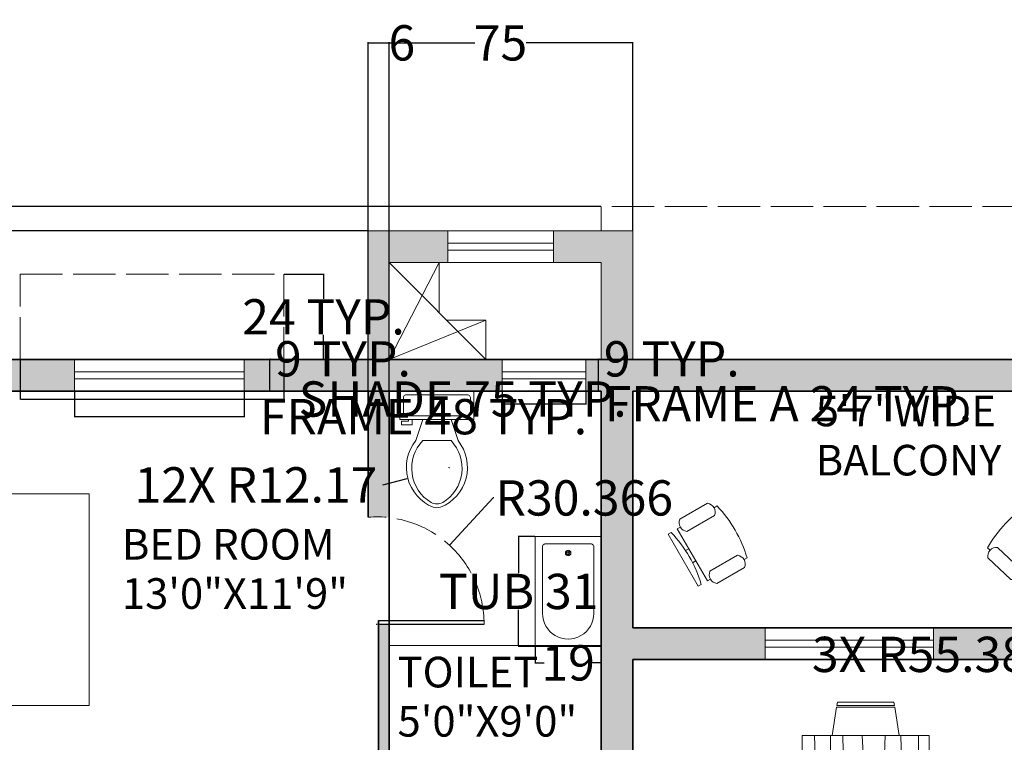
# Model space of a CAD drawing. Units: inches. Extents: x 215 to 969, y -612 to 418.
# Tile 7 of 8: x 405 to 684, y 214 to 418. Entities that reach past the tile are written whole.
import ezdxf

# ---------------------------------------------------------------- set-up
doc = ezdxf.new("R2010")
doc.units = ezdxf.units.IN
doc.header["$MEASUREMENT"] = 0
doc.linetypes.add('ACAD_ISO02W100', pattern=[15, 12, -3])
for name, color, linetype, lineweight in [('A-ANNO-DIMS', 2, 'Continuous', 18), ('A-AREA-IDEN', 7, 'Continuous', 18), ('A-DOOR', 3, 'Continuous', 25), ('A-DOOR-SWNG', 3, 'ACAD_ISO02W100', 13), ('A-FLOR-FIXT', 9, 'Continuous', 18), ('A-FLOR-OVHD', 8, 'ACAD_ISO02W100', 13), ('A-FLOR-SHFT', 9, 'Continuous', 18), ('A-FURN', 8, 'Continuous', 18), ('A-GLAZ', 4, 'Continuous', 18), ('A-WALL', 7, 'Continuous', 35)]:
    doc.layers.add(name, color=color, linetype=linetype, lineweight=lineweight)
doc.layers.add('A-WALL-PATT', color=252, linetype='Continuous', lineweight=13, true_color=0x939598)
doc.styles.get("Standard").update_dxf_attribs({"font": 'arial.ttf'})
doc.dimstyles.get("Standard").update_dxf_attribs({"dimtxt": 10, "dimasz": 0.18, "dimexe": 0.18, "dimexo": 0.0625, "dimgap": 0.09, "dimtad": 0, "dimtih": 1, "dimtoh": 1, "dimdec": 0, "dimzin": 0, "dimdsep": 46, "dimlunit": 3, "dimtxsty": 'Standard', "dimcen": 0.09, "dimadec": 0, "dimazin": 0, "dimtfac": 1, "dimtdec": 0, "dimtofl": 0, "dimtmove": 0, "dimatfit": 3, "dimfxl": 1, "dimtolj": 1, "dimtzin": 0, "dimarcsym": 0})

# ---------------------------------------------------------------- blocks, each defined once
blk = doc.blocks.new('Bed - Queen')
for p, q in [((0, -80.00003), (0, 0)), ((0, 0), (59.99999, 0)), ((59.99999, 0), (59.99999, -80.00003)), ((7.99999, -1.2), (28.79998, -1.2)), ((7.99999, -14.4), (7.99999, -1.2)), ((28.79998, -1.2), (28.79998, -14.4)), ((31.19999, -1.2), (51.99999, -1.2)), ((31.19999, -14.4), (31.19999, -1.2)), ((51.99999, -1.2), (51.99999, -16.4)), ((0, -14.4), (44.8, -14.4)), ((59.99999, -29.6), (44.8, -14.4)), ((44.8, -14.4), (44.8, -29.6)), ((51.99999, -16.4), (46.79936, -16.4)), ((44.8, -16.8), (0, -16.8)), ((44.8, -29.6), (59.99999, -29.6)), ((59.99999, -80.00003), (0, -80.00003))]:
    blk.add_line(p, q)
blk = doc.blocks.new('Dining Set - 36 x 72 in.')
for p, q in [((-22.2343, 26.00059), (-23.4847, 17.99762)), ((-22.2304, 26), (-5.7608, 26)), ((-22, 27.5), (-22.1562, 26.50042)), ((-5.8416, 26.5), (-22.1534, 26.5)), ((-22, 27.5), (-6, 27.5)), ((-5.8437, 26.49966), (-6, 27.5)), ((-4.5152, 17.99762), (-5.7655, 25.99926)), ((5.7657, 26.00059), (4.5153, 17.99762)), ((5.7696, 26), (22.2392, 26)), ((6, 27.5), (5.8438, 26.50042)), ((22.1584, 26.5), (5.8466, 26.5)), ((6, 27.5), (22, 27.5)), ((22.1563, 26.49966), (22, 27.5)), ((23.4848, 17.99762), (22.2345, 25.99926)), ((36, 18), (-36, 18)), ((-36, 18), (-36, -18)), ((36, -18), (36, 18)), ((-44.0006, 8.23428), (-35.9976, 9.48474)), ((44.0006, 8.23428), (35.9976, 9.48474)), ((-45.5, 8), (-44.5004, 8.15617)), ((-45.5, 8), (-45.5, -8)), ((-44.5, -8.15843), (-44.5, 8.15338)), ((-44, 8.23041), (-44, -8.23915)), ((44, 8.23041), (44, -8.23915)), ((44.5, -8.15843), (44.5, 8.15338)), ((45.5, 8), (44.5005, 8.15617)), ((45.5, 8), (45.5, -8)), ((-44.4997, -8.15631), (-45.5, -8)), ((-35.9976, -9.48476), (-43.9993, -8.2345)), ((35.9976, -9.48476), (43.9993, -8.2345)), ((44.4997, -8.15631), (45.5, -8)), ((-36, -18), (36, -18)), ((-22.2343, -26.0006), (-23.4847, -17.99762)), ((-4.5152, -17.99762), (-5.7655, -25.99928)), ((5.7657, -26.0006), (4.5153, -17.99762)), ((23.4848, -17.99762), (22.2345, -25.99928)), ((-22.2304, -26), (-5.7608, -26)), ((-22, -27.5), (-22.1562, -26.50044)), ((-5.8416, -26.5), (-22.1534, -26.5)), ((-22, -27.5), (-6, -27.5)), ((-5.8437, -26.49967), (-6, -27.5)), ((5.7696, -26), (22.2392, -26)), ((6, -27.5), (5.8438, -26.50044)), ((22.1584, -26.5), (5.8466, -26.5)), ((6, -27.5), (22, -27.5)), ((22.1563, -26.49967), (22, -27.5))]:
    blk.add_line(p, q)
for points in [[(-36, 15), (-31.1772, 14.97754), (-26.8079, 14.91406), (-22.8538, 14.81543), (-19.276, 14.6875), (-16.0362, 14.53613), (-13.0957, 14.36718), (-10.4159, 14.18652), (-7.9583, 14), (-5.6904, 13.81315), (-3.6035, 13.63021), (-1.6954, 13.45508), (0.0365, 13.29166), (1.5945, 13.14388), (2.9811, 13.01562), (4.1988, 12.9108), (5.25, 12.83333), (6.1393, 12.78613), (6.8802, 12.76823), (7.4883, 12.77767), (7.9792, 12.8125), (8.3685, 12.87077), (8.6719, 12.95052), (8.9049, 13.0498), (9.0833, 13.16666), (9.2205, 13.29899), (9.3216, 13.44401), (9.3895, 13.59879), (9.4271, 13.76041), (9.4373, 13.92594), (9.4232, 14.09245), (9.3875, 14.257), (9.3333, 14.41666), (9.2638, 14.56917), (9.1836, 14.71484), (9.0975, 14.85465), (9.0104, 14.98958), (8.9272, 15.1206), (8.8529, 15.2487), (8.7922, 15.37483), (8.75, 15.5), (8.7305, 15.62467), (8.7344, 15.74739), (8.7617, 15.86621), (8.8125, 15.97916), (8.8867, 16.08431), (8.9844, 16.17968), (9.1055, 16.26334), (9.25, 16.33333), (9.4189, 16.38802), (9.6172, 16.42708), (9.8506, 16.45052), (10.125, 16.45833), (10.4463, 16.45052), (10.8203, 16.42708), (11.2529, 16.38802), (11.75, 16.33333), (12.3184, 16.26318), (12.9694, 16.17838), (13.7151, 16.07991), (14.5677, 15.96875), (15.5395, 15.84586), (16.6426, 15.71224), (17.8893, 15.56884), (19.2917, 15.41666), (20.859, 15.25667), (22.5879, 15.08984), (24.4721, 14.91715), (26.5052, 14.73958), (28.6809, 14.5581), (30.9929, 14.3737), (33.4347, 14.18733), (36, 14)], [(-36, 10), (-28.9766, 10.14274), (-23.1725, 10.20442), (-18.4241, 10.19775), (-14.5677, 10.13541), (-11.4399, 10.03011), (-8.877, 9.89453), (-6.7154, 9.74137), (-4.7917, 9.58333), (-2.9698, 9.43082), (-1.2246, 9.28515), (0.4415, 9.14534), (2.026, 9.01041), (3.5266, 8.87939), (4.9408, 8.7513), (6.266, 8.62516), (7.5, 8.5), (8.6411, 8.37549), (9.6914, 8.2539), (10.6538, 8.13818), (11.5312, 8.03125), (12.3267, 7.93603), (13.043, 7.85547), (13.6831, 7.79248), (14.25, 7.75), (14.7471, 7.7303), (15.1797, 7.73307), (15.5537, 7.75732), (15.875, 7.80208), (16.1494, 7.86637), (16.3828, 7.94922), (16.5811, 8.04964), (16.75, 8.16666), (16.8944, 8.29915), (17.0143, 8.44531), (17.1089, 8.60319), (17.1771, 8.77083), (17.218, 8.94629), (17.2305, 9.1276), (17.2137, 9.31282), (17.1667, 9.5), (17.0895, 9.6875), (16.987, 9.875), (16.8649, 10.0625), (16.7292, 10.25), (16.5856, 10.4375), (16.4401, 10.625), (16.2985, 10.8125), (16.1667, 11), (16.05, 11.18733), (15.9518, 11.3737), (15.8752, 11.5581), (15.8229, 11.73958), (15.798, 11.91715), (15.8034, 12.08984), (15.842, 12.25667), (15.9167, 12.41666), (16.0295, 12.56836), (16.1784, 12.70833), (16.3605, 12.83268), (16.5729, 12.9375), (16.8127, 13.01888), (17.0768, 13.07291), (17.3625, 13.0957), (17.6667, 13.08333), (17.9894, 13.03312), (18.3418, 12.94726), (18.7382, 12.82918), (19.1927, 12.68229), (19.7195, 12.51001), (20.3327, 12.31575), (21.0465, 12.10294), (21.875, 11.875), (22.8357, 11.63354), (23.959, 11.37304), (25.2786, 11.08618), (26.8282, 10.76562), (28.6414, 10.40405), (30.752, 9.99414), (33.1936, 9.52856), (36, 9)], [(-36, 5.5), (-30.7157, 5.3348), (-26.069, 5.20963), (-21.9946, 5.11767), (-18.4271, 5.05208), (-15.3009, 5.00602), (-12.5508, 4.97265), (-10.1112, 4.94515), (-7.9167, 4.91666), (-5.909, 4.88167), (-4.0586, 4.83984), (-2.3429, 4.79215), (-0.7396, 4.73958), (0.7739, 4.6831), (2.22, 4.6237), (3.6213, 4.56233), (5, 4.5), (6.373, 4.43782), (7.7344, 4.3776), (9.0723, 4.32129), (10.375, 4.27083), (11.6309, 4.22819), (12.8281, 4.19531), (13.9551, 4.17415), (15, 4.16666), (15.954, 4.17448), (16.819, 4.19791), (17.6001, 4.23698), (18.3021, 4.29166), (18.9299, 4.36198), (19.4883, 4.44791), (19.9823, 4.54948), (20.4167, 4.66666), (20.7969, 4.79899), (21.1302, 4.94401), (21.4245, 5.09879), (21.6875, 5.26041), (21.9271, 5.42594), (22.1511, 5.59245), (22.3672, 5.757), (22.5834, 5.91666), (22.8065, 6.06868), (23.0404, 6.21093), (23.2879, 6.34147), (23.5521, 6.45833), (23.8358, 6.55957), (24.142, 6.64323), (24.4735, 6.70735), (24.8334, 6.75), (25.2235, 6.76969), (25.642, 6.76692), (26.0858, 6.74267), (26.5521, 6.69791), (27.0379, 6.63362), (27.5404, 6.55078), (28.0565, 6.45036), (28.5834, 6.33333), (29.1242, 6.19987), (29.7071, 6.04687), (30.3661, 5.87044), (31.1354, 5.66666), (32.0493, 5.43164), (33.142, 5.16146), (34.4475, 4.85221), (36, 4.5)], [(-36, -1), (-30.7915, -0.6591), (-26.0195, -0.38216), (-21.6519, -0.16284), (-17.6563, 0.00521), (-14.0005, 0.12833), (-10.6523, 0.21289), (-7.5796, 0.26522), (-4.75, 0.29166), (-2.134, 0.29793), (0.2878, 0.28711), (2.5317, 0.26163), (4.6146, 0.22396), (6.5529, 0.17651), (8.3633, 0.12174), (10.0623, 0.06209), (11.6667, 0), (13.1899, -0.06201), (14.6341, -0.1211), (15.9982, -0.17432), (17.2813, -0.21875), (18.4823, -0.25147), (19.6003, -0.26953), (20.6343, -0.27002), (21.5834, -0.25), (22.4481, -0.20768), (23.2357, -0.14584), (23.9549, -0.06836), (24.6146, 0.02083), (25.2235, 0.11784), (25.7904, 0.21875), (26.3241, 0.31966), (26.8334, 0.41666), (27.3265, 0.50618), (27.8099, 0.58593), (28.2894, 0.65397), (28.7709, 0.70833), (29.2601, 0.74707), (29.763, 0.76823), (30.2855, 0.76985), (30.8334, 0.75), (31.4088, 0.70784), (31.9994, 0.64713), (32.589, 0.57275), (33.1615, 0.48958), (33.7008, 0.4025), (34.1908, 0.3164), (34.6153, 0.23616), (34.9584, 0.16666), (35.2099, 0.11165), (35.3848, 0.07031), (35.504, 0.04069), (35.5886, 0.02083), (35.6594, 0.00879), (35.7377, 0.0026), (35.8442, 0.00032), (36, 0)], [(-36, -6.5), (-27.1843, -6.31267), (-20.084, -6.1263), (-14.469, -5.9419), (-10.1094, -5.76042), (-6.7752, -5.58285), (-4.2363, -5.41016), (-2.2629, -5.24333), (-0.625, -5.08334), (0.8708, -4.93099), (2.2715, -4.78646), (3.5872, -4.64974), (4.8281, -4.52084), (6.0046, -4.39974), (7.127, -4.28646), (8.2053, -4.18099), (9.25, -4.08334), (10.2705, -3.99382), (11.2734, -3.91407), (12.2647, -3.84603), (13.25, -3.79167), (14.2354, -3.75293), (15.2266, -3.73177), (16.2295, -3.73015), (17.25, -3.75), (18.2912, -3.79248), (19.3451, -3.85547), (20.4009, -3.93604), (21.4479, -4.03125), (22.4754, -4.13819), (23.4727, -4.25391), (24.4289, -4.37549), (25.3334, -4.5), (26.1785, -4.62492), (26.9694, -4.74935), (27.7145, -4.87281), (28.4219, -4.99479), (29.1, -5.11483), (29.7572, -5.23242), (30.4016, -5.34709), (31.0417, -5.45834), (31.6837, -5.56437), (32.3262, -5.65821), (32.9658, -5.73153), (33.599, -5.77604), (34.2224, -5.78345), (34.8327, -5.74545), (35.4264, -5.65373), (36, -5.5)], [(-36, -10), (-26.4022, -9.81299), (-18.4675, -9.62891), (-11.9839, -9.45069), (-6.7396, -9.28125), (-2.5226, -9.12354), (0.8789, -8.98047), (3.6769, -8.85498), (6.0833, -8.75), (8.2767, -8.66765), (10.3021, -8.60677), (12.1712, -8.56543), (13.8958, -8.54167), (15.4876, -8.53353), (16.9583, -8.53907), (18.3197, -8.55632), (19.5834, -8.58334), (20.7616, -8.61841), (21.8685, -8.66081), (22.9188, -8.71004), (23.9271, -8.76563), (24.9081, -8.82707), (25.8763, -8.89388), (26.8465, -8.96558), (27.8334, -9.04167), (28.8474, -9.12118), (29.8828, -9.20117), (30.93, -9.27824), (31.9792, -9.34896), (33.0205, -9.40991), (34.0443, -9.45768), (35.0407, -9.48885), (36, -9.5)], [(-36, -14.5), (-30.0881, -14.33513), (-25.0332, -14.21224), (-20.7312, -14.12647), (-17.0781, -14.07292), (-13.97, -14.04671), (-11.3027, -14.04297), (-8.9724, -14.05681), (-6.875, -14.08334), (-4.9224, -14.11833), (-3.0905, -14.16016), (-1.3709, -14.20785), (0.2448, -14.26042), (1.7647, -14.3169), (3.1973, -14.3763), (4.5507, -14.43767), (5.8333, -14.5), (7.0554, -14.5621), (8.235, -14.62175), (9.3922, -14.67652), (10.5469, -14.72396), (11.7192, -14.76164), (12.929, -14.78711), (14.1965, -14.79794), (15.5417, -14.79167), (16.9933, -14.76424), (18.6152, -14.70508), (20.4804, -14.60197), (22.6615, -14.44271), (25.2312, -14.21509), (28.2624, -13.9069), (31.8277, -13.50594), (36, -13)]]:
    blk.add_lwpolyline(points)
blk = doc.blocks.new('Toilet - top')
for p, q in [((9.5, -6), (9.5, -2)), ((-8, -8.5), (-8, -8)), ((-7, -8), (-7, -9.5)), ((-4, -8), (-6, -14)), ((4, -8), (6, -14)), ((-10, -8.5), (-8, -8.5)), ((-10, -9.5), (-10, -8.5)), ((-7, -9.5), (-10, -9.5)), ((4, -14), (-4, -14))]:
    blk.add_line(p, q)
blk.add_lwpolyline([(10.5, -8), (10.5, 0), (-10.5, 0), (-10.5, -8)], close=True)
for points in [[(-9.5, -2), (-9.5, -6)], [(8.5, -1), (-8.5, -1)], [(-8.5, -7), (8.5, -7)]]:
    blk.add_lwpolyline(points)
for centre, radius, start, end in [((-8.62, -1.88), 0.884, 81.8699, 188.1301), ((8.62, -1.88), 0.884, 351.8699, 98.1301), ((-8.62, -6.12), 0.884, 171.8699, 278.1301), ((8.62, -6.12), 0.884, 261.8699, 8.1301), ((3.52, -21.58), 12.17, 141.4691, 247.9714), ((4.2, -21.82), 11.33, 136.3677, 238.9468), ((-3.52, -21.58), 12.17, 292.0284, 38.5307), ((-4.2, -21.82), 11.33, 301.053, 43.6321), ((0, -27.88), 4, 245.7318, 294.2682), ((0, -29), 4, 254.8605, 285.1395)]:
    blk.add_arc(centre, radius, start, end)
blk = doc.blocks.new('Bath Tub - 26 x 60 in.')
for p, q in [((8, -18), (10, -18)), ((9, -17), (9, -19))]:
    blk.add_line(p, q)
blk.add_lwpolyline([(0, -36), (0, 0), (60, 0), (60, -36)], close=True)
for points in [[(6, -4), (42, -4)], [(4, -30), (4, -6)], [(42, -32), (6, -32)]]:
    blk.add_lwpolyline(points)
for radius in [1.5, 1]:
    blk.add_circle((9, -18), radius)
for centre, radius, start, end in [((5.75, -5.75), 1.77, 81.8699, 188.1301), ((42, -18), 14, 270, 90), ((5.75, -30.25), 1.77, 171.8699, 278.1301)]:
    blk.add_arc(centre, radius, start, end)
blk = doc.blocks.new('Chair - Desk')
for p, q in [((-8.5, 0), (-8.5, -1)), ((-8.5, 0), (8.5, 0)), ((8.5, 0), (8.5, -1)), ((-2, -3), (-2, -1.9355)), ((2, -1.9576), (2, -3)), ((-10.5, -5), (-10.5, -14)), ((-8.5, -3), (-8.5, -4)), ((-8.5, -3), (8.5, -3)), ((-6.5, -14), (-6.5, -5)), ((6.5, -5), (6.5, -14)), ((8.5, -3), (8.5, -4)), ((10.5, -14), (10.5, -5)), ((-8.5, -15), (-8.5, -16)), ((8.5, -15), (8.5, -16))]:
    blk.add_line(p, q)
for centre, radius, start, end in [((0, 34.625), 36.625, 256.5803, 283.4197), ((-8.5, -6.5), 2.5, 36.8699, 143.1301), ((8.5, -6.5), 2.5, 36.8699, 143.1301), ((-8.5, -12.5), 2.5, 216.8699, 323.1301), ((0, 19.625), 36.625, 256.5803, 283.4197), ((8.5, -12.5), 2.5, 216.8699, 323.1301)]:
    blk.add_arc(centre, radius, start, end)
blk = doc.blocks.new('WINDOW-SHADE-75')
for p, q in [((0, 0), (0, 24.15)), ((0, 24.15), (74.66, 24.15)), ((74.66, 24.15), (74.66, 0))]:
    blk.add_line(p, q)
blk = doc.blocks.new('WIN-FRAME-24A')
for p, q in [((0, 0), (0, 9)), ((23.77, 0), (23.77, 9)), ((23.77, 5.5), (0, 5.5)), ((0, 4.5), (0, 0)), ((23.77, 3.5), (0, 3.5))]:
    blk.add_line(p, q)
blk = doc.blocks.new('WIN-FRAME-48')
for p, q in [((0, 4.5), (0, 9)), ((0, 9), (0, 0)), ((48.04, 0), (48.04, 9)), ((48.04, 5.5), (0, 5.5)), ((48.04, 3.5), (0, 3.5))]:
    blk.add_line(p, q)
blk = doc.blocks.new('*D29')
at = {"layer": 'A-ANNO-DIMS', "color": 0, "lineweight": -2, "transparency": 16777216}
for p, q in [((550.61, 272.07), (545.82, 272.07)), ((546, 271.89), (546, 261.7)), ((546, 241.12), (546, 251.3)), ((550.61, 240.94), (545.82, 240.94))]:
    blk.add_line(p, q, dxfattribs=at)
at = {"layer": 'A-ANNO-DIMS', "color": 0, "transparency": 16777216}
for points in [[(545.97, 271.89), (546.03, 271.89), (546, 272.07)], [(545.97, 241.12), (546.03, 241.12), (546, 240.94)]]:
    blk.add_solid(points, dxfattribs=at)
at = {"layer": 'Defpoints', "color": 0, "transparency": 16777216}
for p in [(550.67, 272.07), (546, 240.94), (550.67, 240.94)]:
    blk.add_point(p, dxfattribs=at)
at = {"layer": 'A-ANNO-DIMS', "color": 0, "transparency": 16777216, "insert": (546, 256.5), "char_height": 10, "attachment_point": 5}
blk.add_mtext('\\A1;TUB 31', dxfattribs=at)
blk = doc.blocks.new('*D30')
at = {"layer": 'A-ANNO-DIMS', "color": 0, "lineweight": -2, "transparency": 16777216}
for p, q in [((550.67, 240.87), (550.67, 236.09)), ((569.35, 240.87), (569.35, 236.09)), ((550.85, 236.27), (553.22, 236.27)), ((569.17, 236.27), (566.81, 236.27))]:
    blk.add_line(p, q, dxfattribs=at)
at = {"layer": 'A-ANNO-DIMS', "color": 0, "transparency": 16777216}
for points in [[(550.85, 236.3), (550.85, 236.24), (550.67, 236.27)], [(569.17, 236.3), (569.17, 236.24), (569.35, 236.27)]]:
    blk.add_solid(points, dxfattribs=at)
at = {"layer": 'Defpoints', "color": 0, "transparency": 16777216}
for p in [(550.67, 240.94), (569.35, 240.94), (569.35, 236.27)]:
    blk.add_point(p, dxfattribs=at)
at = {"layer": 'A-ANNO-DIMS', "color": 0, "transparency": 16777216, "insert": (560.01, 236.27), "char_height": 10, "attachment_point": 5}
blk.add_mtext('\\A1;19', dxfattribs=at)
blk = doc.blocks.new('*D45')
at = {"layer": 'A-ANNO-DIMS', "color": 0, "lineweight": -2, "transparency": 16777216}
for p, q in [((541.29, 313.15), (541.29, 309.47)), ((565.06, 313.15), (565.06, 309.47)), ((541.47, 309.65), (564.88, 309.65)), ((565.06, 309.65), (565.24, 309.65))]:
    blk.add_line(p, q, dxfattribs=at)
at = {"layer": 'A-ANNO-DIMS', "color": 0, "transparency": 16777216}
for points in [[(541.47, 309.68), (541.47, 309.62), (541.29, 309.65)], [(564.88, 309.68), (564.88, 309.62), (565.06, 309.65)]]:
    blk.add_solid(points, dxfattribs=at)
at = {"layer": 'Defpoints', "color": 0, "transparency": 16777216}
for p in [(541.29, 313.21), (565.06, 313.21), (565.06, 309.65)]:
    blk.add_point(p, dxfattribs=at)
at = {"layer": 'A-ANNO-DIMS', "color": 0, "transparency": 16777216, "insert": (622.38, 309.65), "char_height": 10, "attachment_point": 5}
blk.add_mtext('\\A1;FRAME A 24 TYP.', dxfattribs=at)
blk = doc.blocks.new('*D46')
at = {"layer": 'A-ANNO-DIMS', "color": 0, "lineweight": -2, "transparency": 16777216}
for p, q in [((565.13, 322.21), (568.81, 322.21)), ((568.63, 322.21), (568.63, 322.39)), ((568.63, 322.39), (568.81, 322.39)), ((568.63, 313.39), (568.63, 322.03)), ((565.13, 313.21), (568.81, 313.21))]:
    blk.add_line(p, q, dxfattribs=at)
at = {"layer": 'A-ANNO-DIMS', "color": 0, "transparency": 16777216}
for points in [[(568.6, 322.03), (568.66, 322.03), (568.63, 322.21)], [(568.6, 313.39), (568.66, 313.39), (568.63, 313.21)]]:
    blk.add_solid(points, dxfattribs=at)
at = {"layer": 'Defpoints', "color": 0, "transparency": 16777216}
for p in [(565.06, 322.21), (568.63, 322.21), (565.06, 313.21)]:
    blk.add_point(p, dxfattribs=at)
at = {"layer": 'A-ANNO-DIMS', "color": 0, "transparency": 16777216, "insert": (589.35, 322.39), "char_height": 10, "attachment_point": 5}
blk.add_mtext('\\A1;9 TYP.', dxfattribs=at)
blk = doc.blocks.new('*D49')
at = {"layer": 'A-ANNO-DIMS', "color": 0, "lineweight": -2, "transparency": 16777216}
for p, q in [((420.28, 313.15), (420.28, 305.83)), ((468.32, 313.15), (468.32, 305.83)), ((420.46, 306.01), (468.14, 306.01)), ((468.32, 306.01), (468.5, 306.01))]:
    blk.add_line(p, q, dxfattribs=at)
at = {"layer": 'A-ANNO-DIMS', "color": 0, "transparency": 16777216}
for points in [[(420.46, 306.04), (420.46, 305.98), (420.28, 306.01)], [(468.14, 306.04), (468.14, 305.98), (468.32, 306.01)]]:
    blk.add_solid(points, dxfattribs=at)
at = {"layer": 'Defpoints', "color": 0, "transparency": 16777216}
for p in [(420.28, 313.21), (468.32, 313.21), (468.32, 306.01)]:
    blk.add_point(p, dxfattribs=at)
at = {"layer": 'A-ANNO-DIMS', "color": 0, "transparency": 16777216, "insert": (519.04, 306.01), "char_height": 10, "attachment_point": 5}
blk.add_mtext('\\A1;FRAME 48 TYP.', dxfattribs=at)
blk = doc.blocks.new('*D50')
at = {"layer": 'A-ANNO-DIMS', "color": 0, "lineweight": -2, "transparency": 16777216}
for p, q in [((468.38, 322.21), (475.71, 322.21)), ((475.53, 322.21), (475.53, 322.39)), ((475.53, 322.39), (475.71, 322.39)), ((475.53, 313.39), (475.53, 322.03)), ((468.38, 313.21), (475.71, 313.21))]:
    blk.add_line(p, q, dxfattribs=at)
at = {"layer": 'A-ANNO-DIMS', "color": 0, "transparency": 16777216}
for points in [[(475.5, 322.03), (475.56, 322.03), (475.53, 322.21)], [(475.5, 313.39), (475.56, 313.39), (475.53, 313.21)]]:
    blk.add_solid(points, dxfattribs=at)
at = {"layer": 'Defpoints', "color": 0, "transparency": 16777216}
for p in [(468.32, 322.21), (475.53, 322.21), (468.32, 313.21)]:
    blk.add_point(p, dxfattribs=at)
at = {"layer": 'A-ANNO-DIMS', "color": 0, "transparency": 16777216, "insert": (496.25, 322.39), "char_height": 10, "attachment_point": 5}
blk.add_mtext('\\A1;9 TYP.', dxfattribs=at)
blk = doc.blocks.new('*D55')
at = {"layer": 'A-ANNO-DIMS', "color": 0, "lineweight": -2, "transparency": 16777216}
for p, q in [((404.88, 322.15), (404.88, 310.83)), ((479.54, 322.15), (479.54, 310.83)), ((405.06, 311.01), (479.36, 311.01)), ((479.54, 311.01), (479.72, 311.01))]:
    blk.add_line(p, q, dxfattribs=at)
at = {"layer": 'A-ANNO-DIMS', "color": 0, "transparency": 16777216}
for points in [[(405.06, 311.04), (405.06, 310.98), (404.88, 311.01)], [(479.36, 311.04), (479.36, 310.98), (479.54, 311.01)]]:
    blk.add_solid(points, dxfattribs=at)
at = {"layer": 'Defpoints', "color": 0, "transparency": 16777216}
for p in [(404.88, 322.21), (479.54, 322.21), (479.54, 311.01)]:
    blk.add_point(p, dxfattribs=at)
at = {"layer": 'A-ANNO-DIMS', "color": 0, "transparency": 16777216, "insert": (530.14, 311.01), "char_height": 10, "attachment_point": 5}
blk.add_mtext('\\A1;SHADE 75 TYP.', dxfattribs=at)
blk = doc.blocks.new('*D56')
at = {"layer": 'A-ANNO-DIMS', "color": 0, "lineweight": -2, "transparency": 16777216}
for p, q in [((479.61, 346.36), (490.92, 346.36)), ((490.74, 346.18), (490.74, 339.4)), ((490.74, 322.39), (490.74, 329.17)), ((479.61, 322.21), (490.92, 322.21))]:
    blk.add_line(p, q, dxfattribs=at)
at = {"layer": 'A-ANNO-DIMS', "color": 0, "transparency": 16777216}
for points in [[(490.71, 346.18), (490.77, 346.18), (490.74, 346.36)], [(490.71, 322.39), (490.77, 322.39), (490.74, 322.21)]]:
    blk.add_solid(points, dxfattribs=at)
at = {"layer": 'Defpoints', "color": 0, "transparency": 16777216}
for p in [(479.54, 346.36), (490.74, 346.36), (479.54, 322.21)]:
    blk.add_point(p, dxfattribs=at)
at = {"layer": 'A-ANNO-DIMS', "color": 0, "transparency": 16777216, "insert": (490.74, 334.29), "char_height": 10, "attachment_point": 5}
blk.add_mtext('\\A1;24 TYP.', dxfattribs=at)
blk = doc.blocks.new('*D76')
at = {"layer": 'A-ANNO-DIMS', "color": 0, "lineweight": -2, "transparency": 16777216}
for p, q in [((569.29, 365.5), (243.77, 365.5)), ((243.95, 365.32), (243.95, -91.71)), ((243.95, -559.13), (243.95, -102.1)), ((454.66, -559.31), (243.77, -559.31))]:
    blk.add_line(p, q, dxfattribs=at)
at = {"layer": 'A-ANNO-DIMS', "color": 0, "transparency": 16777216}
for points in [[(243.92, 365.32), (243.98, 365.32), (243.95, 365.5)], [(243.92, -559.13), (243.98, -559.13), (243.95, -559.31)]]:
    blk.add_solid(points, dxfattribs=at)
at = {"layer": 'Defpoints', "color": 0, "transparency": 16777216}
for p in [(569.35, 365.5), (243.95, -559.31), (454.72, -559.31)]:
    blk.add_point(p, dxfattribs=at)
at = {"layer": 'A-ANNO-DIMS', "color": 0, "transparency": 16777216, "insert": (243.95, -96.91), "char_height": 10, "attachment_point": 5}
blk.add_mtext('\\A1;924.8', dxfattribs=at)
blk = doc.blocks.new('*D77')
at = {"layer": 'A-ANNO-DIMS', "color": 0, "lineweight": -2, "transparency": 16777216}
for p, q in [((503.35, 358.72), (503.35, 412.08)), ((503.53, 411.9), (533.6, 411.9)), ((578.17, 411.9), (548.1, 411.9)), ((578.35, 358.72), (578.35, 412.08))]:
    blk.add_line(p, q, dxfattribs=at)
at = {"layer": 'A-ANNO-DIMS', "color": 0, "transparency": 16777216}
for points in [[(503.53, 411.93), (503.53, 411.87), (503.35, 411.9)], [(578.17, 411.93), (578.17, 411.87), (578.35, 411.9)]]:
    blk.add_solid(points, dxfattribs=at)
at = {"layer": 'Defpoints', "color": 0, "transparency": 16777216}
for p in [(578.35, 411.9), (503.35, 358.66), (578.35, 358.66)]:
    blk.add_point(p, dxfattribs=at)
at = {"layer": 'A-ANNO-DIMS', "color": 0, "transparency": 16777216, "insert": (540.85, 411.9), "char_height": 10, "attachment_point": 5}
blk.add_mtext('\\A1;75', dxfattribs=at)
blk = doc.blocks.new('*D78')
at = {"layer": 'A-ANNO-DIMS', "color": 0, "lineweight": -2, "transparency": 16777216}
for p, q in [((503.29, 358.66), (243.77, 358.66)), ((243.95, 358.48), (243.95, 345.64)), ((243.95, 322.39), (243.95, 335.24)), ((503.29, 322.21), (243.77, 322.21))]:
    blk.add_line(p, q, dxfattribs=at)
at = {"layer": 'A-ANNO-DIMS', "color": 0, "transparency": 16777216}
for points in [[(243.92, 358.48), (243.98, 358.48), (243.95, 358.66)], [(243.92, 322.39), (243.98, 322.39), (243.95, 322.21)]]:
    blk.add_solid(points, dxfattribs=at)
at = {"layer": 'Defpoints', "color": 0, "transparency": 16777216}
for p in [(503.35, 358.66), (243.95, 322.21), (503.35, 322.21)]:
    blk.add_point(p, dxfattribs=at)
at = {"layer": 'A-ANNO-DIMS', "color": 0, "transparency": 16777216, "insert": (243.95, 340.44), "char_height": 10, "attachment_point": 5}
blk.add_mtext('\\A1;36.45', dxfattribs=at)
blk = doc.blocks.new('*D82')
at = {"layer": 'A-ANNO-DIMS', "color": 0, "lineweight": -2, "transparency": 16777216}
for p, q in [((503.35, 313.28), (503.35, 412.08)), ((503.53, 411.9), (509.17, 411.9)), ((509.35, 313.28), (509.35, 412.08)), ((509.35, 411.9), (509.53, 411.9))]:
    blk.add_line(p, q, dxfattribs=at)
at = {"layer": 'A-ANNO-DIMS', "color": 0, "transparency": 16777216}
for points in [[(503.53, 411.93), (503.53, 411.87), (503.35, 411.9)], [(509.17, 411.93), (509.17, 411.87), (509.35, 411.9)]]:
    blk.add_solid(points, dxfattribs=at)
at = {"layer": 'Defpoints', "color": 0, "transparency": 16777216}
for p in [(509.35, 411.9), (503.35, 313.21), (509.35, 313.21)]:
    blk.add_point(p, dxfattribs=at)
at = {"layer": 'A-ANNO-DIMS', "color": 0, "transparency": 16777216, "insert": (512.92, 411.9), "char_height": 10, "attachment_point": 5}
blk.add_mtext('\\A1;6', dxfattribs=at)
blk = doc.blocks.new('*D84')
at = {"layer": 'A-ANNO-DIMS', "color": 0, "lineweight": -2, "transparency": 16777216}
for p, q in [((538.76, 282.99), (526.53, 269.72)), ((538.94, 282.99), (538.76, 282.99)), ((505.74, 247.26), (505.92, 247.26)), ((505.83, 247.17), (505.83, 247.35))]:
    blk.add_line(p, q, dxfattribs=at)
at = {"layer": 'A-ANNO-DIMS', "color": 0, "transparency": 16777216}
blk.add_solid([(526.51, 269.74), (526.55, 269.7), (526.41, 269.59)], dxfattribs=at)
at = {"layer": 'Defpoints', "color": 0, "transparency": 16777216}
for p in [(526.41, 269.59), (505.83, 247.26)]:
    blk.add_point(p, dxfattribs=at)
at = {"layer": 'A-ANNO-DIMS', "color": 0, "transparency": 16777216, "insert": (564.56, 282.99), "char_height": 10, "attachment_point": 5}
blk.add_mtext('\\A1;R30.366', dxfattribs=at)
blk = doc.blocks.new('*D93')
at = {"layer": 'A-ANNO-DIMS', "color": 0, "lineweight": -2, "transparency": 16777216}
for p, q in [((692.12, 238.67), (725.17, 238.67)), ((780.65, 238.67), (780.83, 238.67)), ((780.74, 238.58), (780.74, 238.76))]:
    blk.add_line(p, q, dxfattribs=at)
at = {"layer": 'A-ANNO-DIMS', "color": 0, "transparency": 16777216}
blk.add_solid([(725.17, 238.7), (725.17, 238.64), (725.35, 238.67)], dxfattribs=at)
at = {"layer": 'Defpoints', "color": 0, "transparency": 16777216}
for p in [(725.35, 238.67), (780.74, 238.67)]:
    blk.add_point(p, dxfattribs=at)
at = {"layer": 'A-ANNO-DIMS', "color": 0, "transparency": 16777216, "insert": (659.62, 238.67), "char_height": 10, "attachment_point": 5}
blk.add_mtext('\\A1;3X R55.38', dxfattribs=at)
blk = doc.blocks.new('*D95')
at = {"layer": 'A-ANNO-DIMS', "color": 0, "lineweight": -2, "transparency": 16777216}
for p, q in [((526.28, 291.63), (526.46, 291.63)), ((526.37, 291.54), (526.37, 291.72)), ((507.53, 286.69), (514.42, 288.5))]:
    blk.add_line(p, q, dxfattribs=at)
at = {"layer": 'A-ANNO-DIMS', "color": 0, "transparency": 16777216}
blk.add_solid([(514.41, 288.52), (514.43, 288.47), (514.6, 288.54)], dxfattribs=at)
at = {"layer": 'Defpoints', "color": 0, "transparency": 16777216}
for p in [(526.37, 291.63), (514.6, 288.54)]:
    blk.add_point(p, dxfattribs=at)
at = {"layer": 'A-ANNO-DIMS', "color": 0, "transparency": 16777216, "insert": (471.63, 286.69), "char_height": 10, "attachment_point": 5}
blk.add_mtext('\\A1;12X R12.17', dxfattribs=at)

msp = doc.modelspace()

# ---------------------------------------------------------------- hatches: boundary and pattern name
at = {"layer": 'A-WALL-PATT'}
h = msp.add_hatch(color=256, dxfattribs=at)
h.dxf.hatch_style = 1
h.paths.add_polyline_path([(764.0736, 322.2135), (569.3535, 322.2135), (565.0643, 322.2135), (565.0643, 313.2135), (569.3535, 313.2135), (569.3535, 205.2135), (509.3535, 205.2135), (509.3535, 247.2592), (506.3535, 247.2592), (506.3535, 172.2135), (491.3535, 172.2135), (491.3535, 169.2135), (509.3535, 169.2135), (509.3535, 202.2135), (569.3535, 202.2135), (569.3535, 169.2135), (578.3535, 169.2135), (578.3535, 205.2135), (578.3535, 237.2135), (615.7789, 237.2135), (615.7789, 246.2135), (578.3535, 246.2135), (578.3535, 313.2135), (710.3535, 313.2135), (710.3535, 246.2135), (710.3535, 211.3874), (719.3535, 211.3874), (719.3535, 295.2135), (719.3535, 313.2135), (764.0736, 313.2135)])
h.paths.add_polyline_path([(879.3535, 322.2135), (811.6486, 322.2135), (811.6486, 313.2135), (870.3535, 313.2135), (870.3535, 215.3905, -0.06325422), (879.3535, 216.5337), (879.3535, 313.2135)])
h.paths.add_polyline_path([(879.3535, 157.2135), (879.3535, 180.5337), (870.3535, 180.5337), (870.3535, 157.2135), (719.3535, 157.2135), (710.3535, 157.2135), (710.3535, 148.2135), (719.3535, 148.2135), (870.3535, 148.2135), (870.3535, 16.2135), (838.4933, 16.2135), (838.4933, 13.2135), (870.3535, 13.2135), (870.3535, -37.7865), (844.0345, -37.7865), (844.0345, -46.7865), (870.3535, -46.7865), (879.3535, -46.7865), (879.3535, -37.7865), (879.3535, 137.613)])
h.paths.add_polyline_path([(710.3535, 246.2135), (663.4146, 246.2135), (663.4146, 237.2135), (710.3535, 237.2135)], flags=17)
h.paths.add_polyline_path([(541.2942, 322.2135), (509.3535, 322.2135), (468.3222, 322.2135), (468.3222, 313.2135), (500.3535, 313.2135), (509.3535, 313.2135), (541.2942, 313.2135)])
h.paths.add_polyline_path([(509.3535, 313.2135), (503.3535, 313.2135), (503.3535, 277.5241, -0.04952579), (509.3535, 277.4203)], flags=17)
h.paths.add_polyline_path([(420.2828, 322.2135), (335.3535, 322.2135), (335.3535, 235.2487), (344.3535, 235.2487), (344.3535, 284.1885), (344.3535, 313.2135), (420.2828, 313.2135)])
h.paths.add_polyline_path([(335.3535, 181.2135), (290.3535, 181.2135), (290.3535, 103.2135), (335.3535, 103.2135), (335.3535, 112.2135), (299.3535, 112.2135), (299.3535, 129.1615), (299.3535, 172.2135), (335.3535, 172.2135)])
h.paths.add_polyline_path([(344.3535, 199.3097), (335.3535, 199.3097), (335.3535, 172.2135), (335.3535, 157.3369), (344.3535, 157.3369), (344.3535, 169.2135), (452.3535, 169.2135), (452.5037, 169.2135), (452.5037, 150.1199), (452.3535, 109.2135), (455.3535, 109.2135), (455.3535, 169.2135, -0.02086055), (455.4787, 172.2135), (344.3535, 172.2135)])
h.paths.add_polyline_path([(344.3535, 133.3441), (335.3535, 133.3441), (335.3535, 77.89), (344.3535, 77.89), (344.3535, 103.2135), (401.3556, 103.2135), (401.3556, 109.2135), (344.3535, 109.2135)])
h.paths.add_polyline_path([(462.6362, 109.2135), (443.0437, 109.2135), (425.2018, 109.2135), (425.2018, 106.2135), (452.3535, 106.2135), (462.7615, 106.2135, -0.02086055)])
h.paths.add_polyline_path([(540.3535, 106.2135), (684.3535, 106.2135), (684.3535, 35.7135), (687.3535, 35.7135), (687.3535, 56.1856), (693.3535, 56.1856), (693.3535, 109.2135), (540.3535, 109.2135), (531.3535, 109.2135), (498.6362, 109.2135), (498.6362, 106.2135), (531.3535, 106.2135), (531.3535, -37.7865), (507.9524, -37.7865), (507.9524, -46.7865), (610.6038, -46.7865), (610.6038, -37.7865), (540.3535, -37.7865)])
h.paths.add_polyline_path([(578.3535, 358.6622), (555.879, 358.6622), (555.879, 349.6622), (569.3535, 349.6622), (569.3535, 322.2135), (578.3535, 322.2135)])
h.paths.add_polyline_path([(525.962, 358.6622), (503.3535, 358.6622), (503.3535, 322.2135), (509.3535, 322.2135), (509.3535, 349.6622), (525.962, 349.6622)])
h.paths.add_polyline_path([(344.3535, 30.022), (335.3535, 30.022), (335.3535, -37.7865), (335.3535, -46.7865), (484.3302, -46.7865), (484.3302, -37.7865), (344.3535, -37.7865)])
h.paths.add_polyline_path([(719.1188, -37.7865), (698.4193, -37.7865), (693.3535, -37.7865), (693.3535, 7.424, -0.07717369), (684.3535, 6.0404), (684.3535, -37.7865), (658.8269, -37.7865), (658.8269, -46.7865), (684.3535, -46.7865), (684.3535, -82.7865), (693.3535, -82.7865), (704.1236, -82.7865), (704.1236, -78.0462), (693.3535, -78.0462), (693.3535, -46.7865), (719.1188, -46.7865)])
h.paths.add_polyline_path([(684.3535, -14.2202), (669.6716, -14.2202), (669.6716, -16.6044, -0.23606798), (667.6716, -17.6044), (667.6716, -18.6044, -0.11764706), (650.6716, -18.6044), (650.6716, -17.6044, -0.23606798), (648.6716, -16.6044), (648.6716, -14.2202), (603.0565, -14.2202), (603.0565, -37.7865), (684.3535, -37.7865)], flags=17)
h.paths.add_polyline_path([(665.6716, -14.2202), (652.6716, -14.2202), (652.6716, -16.6044, -0.23606798), (650.6716, -17.6044), (650.6716, -18.6044, 0.11764706), (667.6716, -18.6044), (667.6716, -17.6044, -0.23606798), (665.6716, -16.6044)], flags=16)
h.paths.add_polyline_path([(786.7385, -37.7865), (755.3535, -37.7865), (755.3535, 13.2135), (769.0808, 13.2135), (769.0808, 16.2135), (755.3535, 16.2135), (755.3535, 73.2135), (753.3535, 73.2135), (693.3535, 73.2135), (693.3535, 70.2135), (753.3535, 70.2135), (753.3535, -37.7865), (743.3062, -37.7865), (743.3062, -46.7865), (781.7385, -46.7865), (781.7385, -82.7865), (786.7385, -82.7865), (786.7385, -82.3744), (786.7385, -46.7865)])
h.paths.add_polyline_path([(844.0345, -37.7865), (786.7385, -37.7865), (786.7385, -46.7865), (844.0345, -46.7865)], flags=17)
h.paths.add_polyline_path([(781.7385, -78.0462), (704.1236, -78.0462), (704.1236, -82.7865), (781.7385, -82.7865)], flags=17)
h.paths.add_polyline_path([(344.3535, -46.7865), (335.3535, -46.7865), (335.3535, -166.4525), (344.3535, -166.4525)])
h.paths.add_polyline_path([(382.6632, 103.2135), (344.3535, 103.2135), (344.3535, 77.89), (344.3535, 32.7135), (363.5083, 32.7135), (382.6632, 32.7135)])
h.paths.add_polyline_path([(879.3535, -46.7865), (870.3535, -46.7865), (870.3535, -166.4525), (879.3535, -166.4525)])
h.paths.add_polyline_path([(879.3535, -166.4525), (799.4745, -166.4525), (799.4745, -175.4525), (855.3535, -175.4525), (870.3535, -175.4525), (870.3535, -192.5449), (879.3535, -192.5449), (879.3535, -175.4525)])
h.paths.add_polyline_path([(763.1775, -166.4525), (655.7214, -166.4525), (655.7214, -175.4525), (763.1775, -175.4525)])
h.paths.add_polyline_path([(619.8538, -166.4525), (550.8369, -166.4525), (550.8369, -175.4525), (619.8538, -175.4525)])
h.paths.add_polyline_path([(527.1282, -166.4525), (427.0819, -166.4525), (427.0819, -175.4525), (527.1282, -175.4525)])
h.paths.add_polyline_path([(391.4021, -166.4525), (335.3535, -166.4525), (335.3535, -175.4525), (335.3535, -236.0109), (344.3535, -236.0109), (344.3535, -187.5037), (344.3535, -175.4525), (391.4021, -175.4525)])
h.paths.add_polyline_path([(344.3535, -271.9249), (335.3535, -271.9249), (335.3535, -331.0209), (344.3535, -331.0209), (344.3535, -314.4525), (412.4218, -314.4525, -0.02503209), (412.3073, -311.4525), (344.3535, -311.4525)])
h.paths.add_polyline_path([(470.1954, -311.4525), (442.3073, -311.4525), (442.3073, -314.4525), (470.0702, -314.4525, -0.02086055)])
h.paths.add_polyline_path([(455.3535, -314.4525), (452.3535, -314.4525), (452.3535, -374.4525), (455.3535, -374.4525)])
h.paths.add_polyline_path([(579.3535, -241.4072), (519.3535, -241.4072), (519.3535, -283.4525), (579.3535, -283.4525)])
h.paths.add_polyline_path([(516.5043, -281.1089), (584.3098, -281.1089), (584.3098, -264.0138), (516.5043, -264.0138)], flags=9)
h.paths.add_polyline_path([(516.4662, -263.2183), (581.1504, -263.2183), (581.1504, -245.8948), (516.4662, -245.8948)], flags=9)

# ---------------------------------------------------------------- linework, layer by layer
at = {"layer": 'A-DOOR'}
for p, q in [((506.3535, 247.2592), (506.3535, 248.2592)), ((506.3535, 248.2592), (536.1972, 248.2592)), ((506.3535, 247.2592), (509.3535, 247.2592)), ((506.3535, 247.2592), (536.1972, 247.2592))]:
    msp.add_line(p, q, dxfattribs=at)
at = {"layer": 'A-DOOR-SWNG'}
msp.add_arc((505.8311, 247.2592), 30.3661, 0, 94.680068, dxfattribs=at)
at = {"layer": 'A-FLOR-FIXT'}
msp.add_line((509.3535, 241.2135), (569.3535, 241.2135), dxfattribs=at)
at = {"layer": 'A-FLOR-OVHD'}
for p, q in [((719.3535, 365.5008), (569.3535, 365.5008)), ((569.3535, 365.5008), (569.3535, 358.6622))]:
    msp.add_line(p, q, dxfattribs=at)
at = {"layer": 'A-FLOR-SHFT'}
for p, q in [((578.3535, 358.6622), (503.3535, 358.6622)), ((503.3535, 358.6622), (503.3535, 322.2135)), ((578.3535, 322.2135), (578.3535, 358.6622)), ((509.3535, 322.2135), (509.3535, 349.6622)), ((569.3535, 349.6622), (509.3535, 349.6622)), ((523.5163, 349.6622), (509.3535, 322.2135)), ((509.3535, 349.6622), (536.7306, 322.2135)), ((523.5163, 349.6622), (523.5163, 335.4623)), ((569.3535, 322.2135), (569.3535, 349.6622)), ((509.3535, 322.2135), (536.7306, 333.3094)), ((525.6636, 333.3094), (536.7306, 333.3094)), ((536.7306, 333.3094), (536.7306, 322.2135))]:
    msp.add_line(p, q, dxfattribs=at)
at = {"layer": 'A-GLAZ'}
for p, q in [((525.962, 354.1622), (525.962, 358.6622)), ((525.962, 358.6622), (525.962, 349.6622)), ((555.879, 349.6622), (555.879, 358.6622)), ((555.879, 355.1622), (525.962, 355.1622)), ((555.879, 353.1622), (525.962, 353.1622)), ((615.7789, 246.2135), (615.7789, 237.2135)), ((663.4146, 241.7135), (663.4146, 246.2135)), ((663.4146, 246.2135), (663.4146, 237.2135)), ((615.7789, 242.7135), (663.4146, 242.7135)), ((615.7789, 240.7135), (663.4146, 240.7135))]:
    msp.add_line(p, q, dxfattribs=at)
at = {"layer": 'A-WALL'}
for p, q in [((335.3535, 322.2135), (509.3535, 322.2135)), ((509.3535, 322.2135), (569.3535, 322.2135)), ((569.3535, 322.2135), (879.3535, 322.2135)), ((578.3535, 322.2135), (710.3535, 322.2135)), ((344.3535, 313.2135), (500.3535, 313.2135)), ((500.3535, 313.2135), (509.3535, 313.2135)), ((503.3535, 277.6208), (503.3535, 313.2135)), ((509.3535, 313.2135), (569.3535, 313.2135)), ((509.3535, 205.2135), (509.3535, 313.2135)), ((569.3535, 313.2135), (569.3535, 205.2135)), ((578.3535, 313.2135), (578.3535, 246.2135)), ((578.3535, 313.2135), (710.3535, 313.2135)), ((503.3535, 277.6208), (503.3535, 277.5241)), ((506.3535, 172.2135), (506.3535, 248.2592)), ((710.3535, 246.2135), (578.3535, 246.2135)), ((710.3535, 237.2135), (578.3535, 237.2135)), ((578.3535, 237.2135), (578.3535, 205.2135))]:
    msp.add_line(p, q, dxfattribs=at)

# ---------------------------------------------------------------- block references
at = {"layer": 'A-FLOR-FIXT'}
msp.add_blockref('Toilet - top', (522.8465, 313.2135), dxfattribs=at)
at = {"layer": 'A-FLOR-FIXT', "xscale": 0.5188855391372424, "yscale": 0.5188855391372424, "zscale": 0.5188855391372424, "rotation": 270}
msp.add_blockref('Bath Tub - 26 x 60 in.', (569.3535, 272.0698), dxfattribs=at)
at = {"layer": 'A-FLOR-OVHD'}
msp.add_blockref('WINDOW-SHADE-75', (404.8838, 322.214), dxfattribs=at)
at = {"layer": 'A-FURN'}
for name, p, rotation in [('Bed - Queen', (344.3535, 224.1885), 90), ('Chair - Desk', (592.5744, 265.3678), 119.9999999999999), ('Chair - Desk', (696.2113, 264.0519), 226.5917899333866), ('Dining Set - 36 x 72 in.', (644.2464, 179.6732), 270)]:
    msp.add_blockref(name, p, dxfattribs=dict(at, rotation=rotation))
at = {"layer": 'A-GLAZ'}
for name, p in [('WIN-FRAME-48', (420.283, 313.214)), ('WIN-FRAME-24A', (541.294, 313.214))]:
    msp.add_blockref(name, p, dxfattribs=at)

# ---------------------------------------------------------------- texts
at = {"layer": 'A-AREA-IDEN'}
for s, height, p in [('5\'7"WIDE', 8.67737, (630.1052, 303.2851)), ('BALCONY', 8.67737, (630.1052, 289.3457)), ('BED ROOM', 8.67737, (433.6724, 265.511)), ('13\'0"X11\'9"', 8.677368, (433.6724, 251.5716)), ('TOILET', 8.67737, (511.7108, 229.3177)), ('5\'0"X9\'0"', 8.67737, (511.7108, 215.3783))]:
    msp.add_text(s, height=height, dxfattribs=at).set_placement(p)

# ---------------------------------------------------------------- dimensions: what is measured, and where the dimension line sits
at = {"layer": 'A-ANNO-DIMS'}
for base, p1, p2, picture, middle in [((578.3535, 411.9008), (503.3535, 358.6622), (578.3535, 358.6622), '*D77', (540.8535, 411.9008)), ((509.3535, 411.9008), (503.3535, 313.2135), (509.3535, 313.2135), '*D82', (512.925, 411.9008)), ((569.3535, 236.2667), (550.6736, 240.9367), (569.3535, 240.9367), '*D30', (560.0136, 236.2667))]:
    dim = msp.add_linear_dim(base=base, p1=p1, p2=p2, dimstyle='Standard', override={"dimdec": 0, "dimlfac": 1, "dimrnd": 0, "dimzin": 0, "dimdsep": 46, "dimlunit": 2}, dxfattribs=at)
    dim.commit()
    dim.dimension.update_dxf_attribs({"geometry": picture, "text_midpoint": middle})
for base, p1, p2, override, picture, middle in [((243.9535, -559.3132), (569.3535, 365.5008), (454.7218, -559.3132), {"dimdec": 1, "dimlfac": 1, "dimrnd": 0, "dimzin": 0, "dimdsep": 46, "dimlunit": 2}, '*D76', (243.9535, -96.9062)), ((243.9535, 322.2135), (503.3535, 358.6622), (503.3535, 322.2135), {"dimdec": 2, "dimlfac": 1, "dimrnd": 0, "dimzin": 0, "dimdsep": 46, "dimlunit": 2}, '*D78', (243.9535, 340.4379))]:
    dim = msp.add_linear_dim(base=base, p1=p1, p2=p2, angle=90, dimstyle='Standard', override=override, dxfattribs=at)
    dim.commit()
    dim.dimension.update_dxf_attribs({"geometry": picture, "text_midpoint": middle})
for base, p1, p2, angle, text, picture, middle in [((490.7439, 346.3623), (479.5447, 322.2135), (479.5447, 346.3623), 90, '<> TYP.', '*D56', (490.7439, 334.2879)), ((475.5281, 322.2135), (468.3222, 313.2135), (468.3222, 322.2135), 90, '<> TYP.', '*D50', (496.2517, 322.3935)), ((568.6298, 322.2135), (565.0643, 313.2135), (565.0643, 322.2135), 90, '<> TYP.', '*D46', (589.3534, 322.3935)), ((546.0036, 240.9367), (550.6736, 272.0698), (550.6736, 240.9367), 270, 'TUB <>', '*D29', (546.0036, 256.5033))]:
    dim = msp.add_linear_dim(base=base, p1=p1, p2=p2, angle=angle, text=text, dimstyle='Standard', override={"dimdec": 0, "dimlfac": 1, "dimrnd": 0, "dimzin": 0, "dimdsep": 46, "dimlunit": 2}, dxfattribs=at)
    dim.commit()
    dim.dimension.update_dxf_attribs({"geometry": picture, "text_midpoint": middle})
for base, p1, p2, text, picture, middle in [((565.0643, 309.648), (541.2942, 313.2135), (565.0643, 313.2135), 'FRAME A <> TYP.', '*D45', (622.3772, 309.648)), ((479.5447, 311.0143), (404.8833, 322.2135), (479.5447, 322.2135), 'SHADE <> TYP.', '*D55', (530.1353, 311.0143)), ((468.3222, 306.0076), (420.2828, 313.2135), (468.3222, 313.2135), 'FRAME <> TYP.', '*D49', (519.0356, 306.0076))]:
    dim = msp.add_linear_dim(base=base, p1=p1, p2=p2, text=text, dimstyle='Standard', override={"dimdec": 0, "dimlfac": 1, "dimrnd": 0, "dimzin": 0, "dimdsep": 46, "dimlunit": 2}, dxfattribs=at)
    dim.commit()
    dim.dimension.update_dxf_attribs({"geometry": picture, "text_midpoint": middle})
for center, mpoint, text, picture, middle in [((526.3661, 291.6331), (514.5964, 288.5411), '12X <>', '*D95', (507.5346, 286.6859)), ((780.7379, 238.6687), (725.3534, 238.669), '3X <>', '*D93', (692.1228, 238.6692))]:
    dim = msp.add_radius_dim(center=center, mpoint=mpoint, text=text, dimstyle='Standard', override={"dimdec": 2, "dimlfac": 1, "dimrnd": 0, "dimzin": 0, "dimdsep": 46, "dimlunit": 2}, dxfattribs=at)
    dim.commit()
    dim.dimension.update_dxf_attribs({"geometry": picture, "text_midpoint": middle, "dimtype": 164})
dim = msp.add_radius_dim(center=(505.8311, 247.2592), mpoint=(526.4088, 269.5898), dimstyle='Standard', override={"dimdec": 3, "dimlfac": 1, "dimrnd": 0, "dimzin": 0, "dimdsep": 46, "dimlunit": 2}, dxfattribs=at)
dim.commit()
dim.dimension.update_dxf_attribs({"geometry": '*D84', "text_midpoint": (564.5644, 282.9882), "dimtype": 164})

doc.saveas('drawing.dxf')
